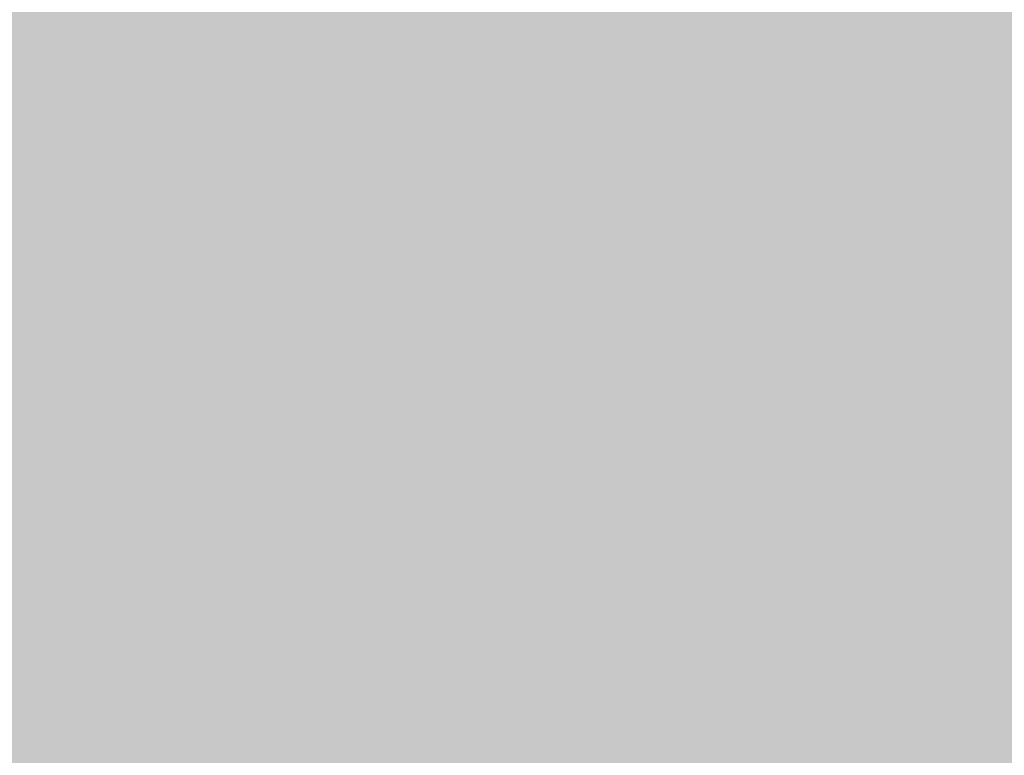
# Model space of a CAD drawing. Units: feet. Extents: x 3168 to 4724, y 827 to 1477.
# Tile 27 of 256: x 3261.901 to 3270.273, y 1087.401 to 1093.654. Entities that reach past the tile are written whole.
import ezdxf

# ---------------------------------------------------------------- set-up
doc = ezdxf.new("R2010")
doc.units = ezdxf.units.FT
doc.layers.add('A-ELEV-PATT', color=8, linetype='Continuous', lineweight=13)

msp = doc.modelspace()

# ---------------------------------------------------------------- hatches: boundary and pattern name
at = {"layer": 'A-ELEV-PATT'}
h = msp.add_hatch(color=256, dxfattribs=at)
h.dxf.hatch_style = 1
edge = h.paths.add_edge_path()
edge.add_ellipse((3552.9058, 979.2201), major_axis=(36.7449, 0), ratio=0.4848485, start_angle=0, end_angle=360)
edge = h.paths.add_edge_path()
edge.add_ellipse((3559.8916, 929.2523), major_axis=(36.7449, 0), ratio=0.4848485, start_angle=0, end_angle=360)
edge = h.paths.add_edge_path()
edge.add_line((3299.3168, 1198.6061), (3479.9167, 1198.6061))
edge.add_line((3479.9167, 1198.6061), (3479.9167, 1209.8686))
edge.add_spline(control_points=[(3479.9167, 1209.8686), (3464.3012, 1209.8686), (3448.6856, 1209.8686), (3410.9491, 1209.8686), (3388.8282, 1209.8686), (3355.6469, 1209.8686), (3344.5864, 1209.8686), (3327.9957, 1209.8686), (3322.4655, 1209.8686), (3314.1702, 1209.8686), (3311.4051, 1209.8686), (3307.2574, 1209.8686), (3305.8748, 1209.8686), (3303.801, 1209.8686), (3303.1097, 1209.8686), (3302.0728, 1209.8686), (3301.7272, 1209.8686), (3301.2087, 1209.8686), (3301.0359, 1209.8686), (3300.7767, 1209.8686), (3300.6903, 1209.8686), (3300.5606, 1209.8686), (3300.5174, 1209.8686), (3300.4526, 1209.8686), (3300.431, 1209.8686), (3300.3986, 1209.8686), (3300.3878, 1209.8686), (3300.3662, 1209.8686), (3300.3457, 1209.8686), (3300.3455, 1209.8686), (3300.3455, 1209.8686), (3300.3433, 1209.8686), (3300.3411, 1209.8686), (3300.3379, 1209.8686), (3300.3368, 1209.8686), (3300.3339, 1209.8686), (3300.3321, 1209.8686), (3300.3255, 1209.8686), (3300.3207, 1209.8686), (3300.3109, 1209.8686), (3300.306, 1209.8686), (3300.2905, 1209.8686), (3300.28, 1209.8686), (3300.2324, 1209.8688), (3300.1953, 1209.869), (3299.9511, 1209.8706), (3299.7448, 1209.8743), (3299.4368, 1209.8833), (3299.3344, 1209.8868), (3299.1811, 1209.8929), (3299.13, 1209.8951), (3298.6522, 1209.9168), (3298.2295, 1209.9457), (3297.6016, 1210.0024), (3297.3934, 1210.0235), (3297.0827, 1210.0583), (3296.9793, 1210.0705), (3296.293, 1210.1549), (3295.7181, 1210.2434), (3294.8687, 1210.3989), (3294.5877, 1210.4545), (3294.1693, 1210.5433), (3294.0304, 1210.5739), (3291.7071, 1211.1012), (3289.6536, 1211.8134), (3285.7763, 1213.564), (3283.9514, 1214.6035), (3280.5122, 1216.9801), (3278.8972, 1218.3176), (3276.3799, 1220.8295), (3275.416, 1221.9177), (3274.0393, 1223.7077), (3273.581, 1224.3495), (3273.1432, 1225.0163)], knot_values=[39.119033, 39.119033, 39.119033, 39.119033, 39.286353, 39.286353, 39.523379, 39.523379, 39.641892, 39.641892, 39.701148, 39.701148, 39.730777, 39.730777, 39.745591, 39.745591, 39.752998, 39.752998, 39.756701, 39.756701, 39.758553, 39.758553, 39.759479, 39.759479, 39.759942, 39.759942, 39.760173, 39.760173, 39.760289, 39.760289, 39.760405, 39.760405, 39.760463, 39.760463, 39.763389, 39.763389, 39.764851, 39.764851, 39.767304, 39.767304, 39.773825, 39.773825, 39.78057, 39.78057, 39.79477, 39.79477, 39.845194, 39.845194, 40.126715, 40.126715, 40.267476, 40.267476, 40.337856, 40.337856, 40.927023, 40.927023, 41.221606, 41.221606, 41.368898, 41.368898, 42.202622, 42.202622, 42.619485, 42.619485, 42.827916, 42.827916, 46.118323, 46.118323, 49.408731, 49.408731, 52.699139, 52.699139, 54.927489, 54.927489, 56.104228, 56.104228, 56.104228, 56.104228], weights=[1, 1, 1, 1, 1, 1, 1, 1, 1, 1, 1, 1, 1, 1, 1, 1, 1, 1, 1, 1, 1, 1, 1, 1, 1, 1, 1, 1, 1, 1, 1, 1, 1, 1, 1, 1, 1, 1, 1, 1, 1, 1, 1, 1, 1, 1, 1, 1, 1, 1, 1, 1, 1, 1, 1, 1, 1, 1, 1, 1, 1, 1, 1, 1, 1, 1, 1, 1, 1, 1, 1, 1, 1, 1], degree=3, periodic=0)
edge.add_line((3273.1432, 1225.0163), (3273.1432, 1099.0163))
edge.add_line((3273.1432, 1099.0163), (3299.3168, 1099.0163))
edge.add_line((3299.3168, 1099.0163), (3299.3168, 1198.6061))
edge = h.paths.add_edge_path()
edge.add_line((3304.7584, 1324.1581), (3479.9167, 1324.1581))
edge.add_line((3479.9167, 1324.1581), (3479.9167, 1335.7146))
edge.add_line((3479.9167, 1335.7146), (3269.1616, 1335.7146))
edge.add_spline(control_points=[(3269.1616, 1335.7146), (3264.0242, 1335.7146), (3258.3641, 1328.9582), (3259.2643, 1323.9003)], knot_values=[0, 0, 0, 0, 15.412191, 15.412191, 15.412191, 15.412191], degree=3, periodic=0)
edge.add_line((3259.2643, 1323.9003), (3265.5168, 1288.7691))
edge.add_line((3265.5168, 1288.7691), (3275.2651, 1261.5456))
edge.add_line((3275.2651, 1261.5456), (3304.7584, 1261.5456))
edge.add_line((3304.7584, 1261.5456), (3304.7584, 1324.1581))
h = msp.add_hatch(color=256, dxfattribs=at)
h.dxf.hatch_style = 1
h.paths.add_polyline_path([(3384.5252, 1099.0163), (3335.0292, 1099.0163), (3299.3168, 1099.0163), (3273.1432, 1099.0163), (3217.5654, 1099.0163), (3168.0693, 827.1163), (3335.0292, 827.1163)])

doc.saveas('drawing.dxf')
